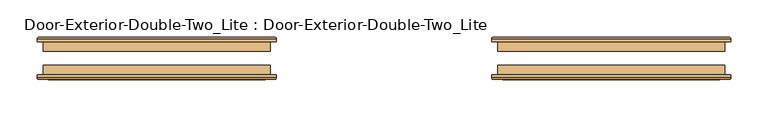
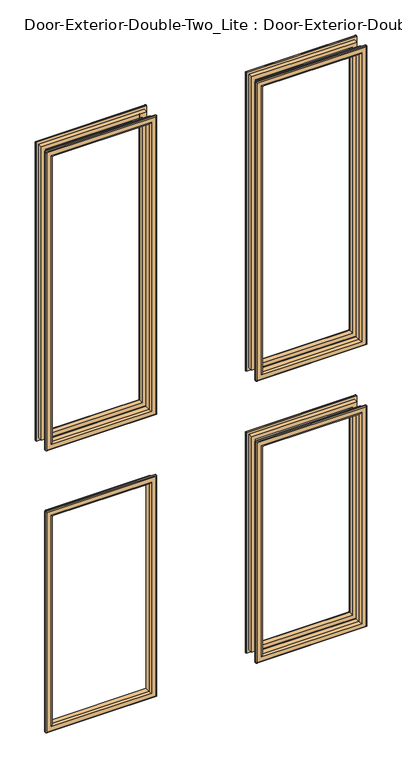
"""IFC4 building model written with IfcOpenShell, lengths in millimetres: door geometry, Door-Exterior-Double-Two_Lite : Door-Exterior-Double-Two_Lite."""

from ifc_helpers import new_model, si_unit, frame, origin, place, context, project, spatial, ellipse_curve, source, transform, mapped, element, save
from ifc_brep_helpers import plane_surface, cylinder_surface, advanced_brep


def door_exterior_double_two_lite_door_exterior_double_two_lite_31e28e64(model_context):
    return source(origin(), model_context, "Body", "AdvancedBrep", [
        advanced_brep(
        [(-457.2, 63.5, 1117.6), (-457.2, 50.8, 1117.6), (-457.2, 50.8, 2016.125), (-457.2, 63.5, 2016.125), (-445.2, 49.8, 1129.6), (-445.2, 63.5, 1129.6), (-445.2, 63.5, 2004.125), (-445.2, 49.8, 2004.125), (-450.2, 44.8, 1124.6), (-450.2, 44.8, 2009.125), (-465.2, 46.8, 1109.6), (-463.2, 44.8, 1111.6), (-463.2, 44.8, 2022.125), (-465.2, 46.8, 2024.125), (-465.2, 50.8, 1109.6), (-465.2, 50.8, 2024.125), (-152.4, 50.8, 2016.125), (-152.4, 63.5, 2016.125), (-164.4, 63.5, 2004.125), (-164.4, 49.8, 2004.125), (-159.4, 44.8, 2009.125), (-146.4, 44.8, 2022.125), (-144.4, 46.8, 2024.125), (-144.4, 50.8, 2024.125), (-152.4, 50.8, 1117.6), (-152.4, 63.5, 1117.6), (-164.4, 63.5, 1129.6), (-164.4, 49.8, 1129.6), (-159.4, 44.8, 1124.6), (-146.4, 44.8, 1111.6), (-144.4, 46.8, 1109.6), (-144.4, 50.8, 1109.6)],
        [
            (0, 1),
            (1, 2),
            (2, 3),
            (3, 0),
            (4, 5),
            (5, 6),
            (6, 7),
            (7, 4),
            (8, 4, ellipse_curve(frame((-450.2, 49.8, 1124.6), z_axis=(-0.7071067811865475, 0.0, 0.7071067811865475), x_axis=(-0.7071067811865474, 0.0, -0.7071067811865476)), 7.0710678, 5.0)),
            (7, 9, ellipse_curve(frame((-450.2, 49.8, 2009.125), z_axis=(-0.7071067811865475, 0.0, -0.7071067811865475), x_axis=(0.7071067811865474, 0.0, -0.7071067811865476)), 7.0710678, 5.0)),
            (9, 8),
            (10, 11, ellipse_curve(frame((-463.2, 46.8, 1111.6), z_axis=(-0.7071067811865475, 0.0, 0.7071067811865475), x_axis=(-0.7071067811865474, 0.0, -0.7071067811865476)), 2.8284271, 2.0)),
            (11, 12),
            (12, 13, ellipse_curve(frame((-463.2, 46.8, 2022.125), z_axis=(-0.7071067811865475, 0.0, -0.7071067811865475), x_axis=(0.7071067811865474, 0.0, -0.7071067811865476)), 2.8284271, 2.0)),
            (13, 10),
            (14, 10),
            (13, 15),
            (15, 14),
            (2, 16),
            (16, 17),
            (17, 3),
            (6, 18),
            (18, 19),
            (19, 7),
            (19, 20, ellipse_curve(frame((-159.4, 49.8, 2009.125), z_axis=(-0.7071067811865475, 0.0, 0.7071067811865475), x_axis=(-0.7071067811865476, 0.0, -0.7071067811865474)), 7.0710678, 5.0)),
            (20, 9),
            (12, 21),
            (21, 22, ellipse_curve(frame((-146.4, 46.8, 2022.125), z_axis=(-0.7071067811865475, 0.0, 0.7071067811865475), x_axis=(-0.7071067811865476, 0.0, -0.7071067811865474)), 2.8284271, 2.0)),
            (22, 13),
            (22, 23),
            (23, 15),
            (16, 24),
            (24, 25),
            (25, 17),
            (18, 26),
            (26, 27),
            (27, 19),
            (27, 28, ellipse_curve(frame((-159.4, 49.8, 1124.6), z_axis=(0.7071067811865475, 0.0, 0.7071067811865475), x_axis=(-0.7071067811865474, 0.0, 0.7071067811865476)), 7.0710678, 5.0)),
            (28, 20),
            (21, 29),
            (29, 30, ellipse_curve(frame((-146.4, 46.8, 1111.6), z_axis=(0.7071067811865475, 0.0, 0.7071067811865475), x_axis=(-0.7071067811865474, 0.0, 0.7071067811865476)), 2.8284271, 2.0)),
            (30, 22),
            (30, 31),
            (31, 23),
            (31, 14),
            (1, 24),
            (0, 25),
            (5, 26),
            (4, 27),
            (8, 28),
            (11, 29),
            (10, 30),
        ],
        [
            plane_surface(frame((-457.2, 50.8, 1117.6), z_axis=(-1.0, 0.0, 0.0), x_axis=(0.0, 0.0, 1.0))),
            plane_surface(frame((-445.2, 63.5, 1129.6), z_axis=(1.0, 0.0, 0.0), x_axis=(0.0, 0.0, 1.0))),
            cylinder_surface(frame((-450.2, 49.8, 1117.6), z_axis=(0.0, 0.0, -1.0), x_axis=(-1.0, 0.0, 0.0)), 5.0),
            cylinder_surface(frame((-463.2, 46.8, 1117.6), z_axis=(0.0, 0.0, -1.0), x_axis=(-1.0, 0.0, 0.0)), 2.0),
            plane_surface(frame((-465.2, 46.8, 1109.6), z_axis=(-1.0, 0.0, 0.0), x_axis=(0.0, 0.0, 1.0))),
            plane_surface(frame((-457.2, 50.8, 2016.125), z_axis=(0.0, 0.0, 1.0), x_axis=(1.0, 0.0, 0.0))),
            plane_surface(frame((-445.2, 63.5, 2004.125), z_axis=(0.0, 0.0, -1.0), x_axis=(1.0, 0.0, 0.0))),
            cylinder_surface(frame((-457.2, 49.8, 2009.125), z_axis=(-1.0, 0.0, 0.0), x_axis=(0.0, 0.0, 1.0)), 5.0),
            cylinder_surface(frame((-457.2, 46.8, 2022.125), z_axis=(-1.0, 0.0, 0.0), x_axis=(0.0, 0.0, 1.0)), 2.0),
            plane_surface(frame((-465.2, 46.8, 2024.125), z_axis=(0.0, 0.0, 1.0), x_axis=(1.0, 0.0, 0.0))),
            plane_surface(frame((-152.4, 50.8, 2016.125), z_axis=(1.0, 0.0, 0.0), x_axis=(0.0, 0.0, -1.0))),
            plane_surface(frame((-164.4, 63.5, 2004.125), z_axis=(-1.0, 0.0, 0.0), x_axis=(0.0, 0.0, -1.0))),
            cylinder_surface(frame((-159.4, 49.8, 2016.125), z_axis=(0.0, 0.0, 1.0), x_axis=(1.0, 0.0, 0.0)), 5.0),
            cylinder_surface(frame((-146.4, 46.8, 2016.125), z_axis=(0.0, 0.0, 1.0), x_axis=(1.0, 0.0, 0.0)), 2.0),
            plane_surface(frame((-144.4, 46.8, 2024.125), z_axis=(1.0, 0.0, 0.0), x_axis=(0.0, 0.0, -1.0))),
            plane_surface(frame((-144.4, 50.8, 1109.6), z_axis=(0.0, 1.0, 0.0), x_axis=(-1.0, 0.0, 0.0))),
            plane_surface(frame((-152.4, 50.8, 1117.6), z_axis=(0.0, 0.0, -1.0), x_axis=(-1.0, 0.0, 0.0))),
            plane_surface(frame((-152.4, 63.5, 1117.6), z_axis=(0.0, 1.0, 0.0), x_axis=(-1.0, 0.0, 0.0))),
            plane_surface(frame((-164.4, 63.5, 1129.6), z_axis=(0.0, 0.0, 1.0), x_axis=(-1.0, 0.0, 0.0))),
            cylinder_surface(frame((-152.4, 49.8, 1124.6), z_axis=(1.0, 0.0, 0.0), x_axis=(0.0, 0.0, -1.0)), 5.0),
            plane_surface(frame((-159.4, 44.8, 1124.6), z_axis=(0.0, -1.0, 0.0), x_axis=(-1.0, 0.0, 0.0))),
            cylinder_surface(frame((-152.4, 46.8, 1111.6), z_axis=(1.0, 0.0, 0.0), x_axis=(0.0, 0.0, -1.0)), 2.0),
            plane_surface(frame((-144.4, 46.8, 1109.6), z_axis=(0.0, 0.0, -1.0), x_axis=(-1.0, 0.0, 0.0))),
        ],
        [
            (0, [[1, 2, 3, 4]]),
            (1, [[5, 6, 7, 8]]),
            (2, [[9, -8, 10, 11]]),
            (3, [[12, 13, 14, 15]]),
            (4, [[16, -15, 17, 18]]),
            (5, [[-3, 19, 20, 21]]),
            (6, [[-7, 22, 23, 24]]),
            (7, [[-10, -24, 25, 26]]),
            (8, [[-14, 27, 28, 29]]),
            (9, [[-17, -29, 30, 31]]),
            (10, [[-20, 32, 33, 34]]),
            (11, [[-23, 35, 36, 37]]),
            (12, [[-25, -37, 38, 39]]),
            (13, [[-28, 40, 41, 42]]),
            (14, [[-30, -42, 43, 44]]),
            (15, [[-31, -44, 45, -18], [46, -32, -19, -2]]),
            (16, [[-33, -46, -1, 47]]),
            (17, [[-21, -34, -47, -4], [48, -35, -22, -6]]),
            (18, [[-36, -48, -5, 49]]),
            (19, [[-38, -49, -9, 50]]),
            (20, [[51, -40, -27, -13], [-26, -39, -50, -11]]),
            (21, [[-41, -51, -12, 52]]),
            (22, [[-43, -52, -16, -45]]),
        ],
    ),
        advanced_brep(
        [(152.4, 63.5, 1117.6), (152.4, 50.8, 1117.6), (152.4, 50.8, 2016.125), (152.4, 63.5, 2016.125), (164.4, 49.8, 1129.6), (164.4, 63.5, 1129.6), (164.4, 63.5, 2004.125), (164.4, 49.8, 2004.125), (159.4, 44.8, 1124.6), (159.4, 44.8, 2009.125), (144.4, 46.8, 1109.6), (146.4, 44.8, 1111.6), (146.4, 44.8, 2022.125), (144.4, 46.8, 2024.125), (144.4, 50.8, 1109.6), (144.4, 50.8, 2024.125), (457.2, 50.8, 2016.125), (457.2, 63.5, 2016.125), (445.2, 63.5, 2004.125), (445.2, 49.8, 2004.125), (450.2, 44.8, 2009.125), (463.2, 44.8, 2022.125), (465.2, 46.8, 2024.125), (465.2, 50.8, 2024.125), (457.2, 50.8, 1117.6), (457.2, 63.5, 1117.6), (445.2, 63.5, 1129.6), (445.2, 49.8, 1129.6), (450.2, 44.8, 1124.6), (463.2, 44.8, 1111.6), (465.2, 46.8, 1109.6), (465.2, 50.8, 1109.6)],
        [
            (0, 1),
            (1, 2),
            (2, 3),
            (3, 0),
            (4, 5),
            (5, 6),
            (6, 7),
            (7, 4),
            (8, 4, ellipse_curve(frame((159.4, 49.8, 1124.6), z_axis=(-0.7071067811865475, 0.0, 0.7071067811865475), x_axis=(-0.7071067811865474, 0.0, -0.7071067811865476)), 7.0710678, 5.0)),
            (7, 9, ellipse_curve(frame((159.4, 49.8, 2009.125), z_axis=(-0.7071067811865475, 0.0, -0.7071067811865475), x_axis=(0.7071067811865474, 0.0, -0.7071067811865476)), 7.0710678, 5.0)),
            (9, 8),
            (10, 11, ellipse_curve(frame((146.4, 46.8, 1111.6), z_axis=(-0.7071067811865475, 0.0, 0.7071067811865475), x_axis=(-0.7071067811865474, 0.0, -0.7071067811865476)), 2.8284271, 2.0)),
            (11, 12),
            (12, 13, ellipse_curve(frame((146.4, 46.8, 2022.125), z_axis=(-0.7071067811865475, 0.0, -0.7071067811865475), x_axis=(0.7071067811865474, 0.0, -0.7071067811865476)), 2.8284271, 2.0)),
            (13, 10),
            (14, 10),
            (13, 15),
            (15, 14),
            (2, 16),
            (16, 17),
            (17, 3),
            (6, 18),
            (18, 19),
            (19, 7),
            (19, 20, ellipse_curve(frame((450.2, 49.8, 2009.125), z_axis=(-0.7071067811865475, 0.0, 0.7071067811865475), x_axis=(-0.7071067811865476, 0.0, -0.7071067811865474)), 7.0710678, 5.0)),
            (20, 9),
            (12, 21),
            (21, 22, ellipse_curve(frame((463.2, 46.8, 2022.125), z_axis=(-0.7071067811865475, 0.0, 0.7071067811865475), x_axis=(-0.7071067811865476, 0.0, -0.7071067811865474)), 2.8284271, 2.0)),
            (22, 13),
            (22, 23),
            (23, 15),
            (16, 24),
            (24, 25),
            (25, 17),
            (18, 26),
            (26, 27),
            (27, 19),
            (27, 28, ellipse_curve(frame((450.2, 49.8, 1124.6), z_axis=(0.7071067811865475, 0.0, 0.7071067811865475), x_axis=(-0.7071067811865474, 0.0, 0.7071067811865476)), 7.0710678, 5.0)),
            (28, 20),
            (21, 29),
            (29, 30, ellipse_curve(frame((463.2, 46.8, 1111.6), z_axis=(0.7071067811865475, 0.0, 0.7071067811865475), x_axis=(-0.7071067811865474, 0.0, 0.7071067811865476)), 2.8284271, 2.0)),
            (30, 22),
            (30, 31),
            (31, 23),
            (31, 14),
            (1, 24),
            (0, 25),
            (5, 26),
            (4, 27),
            (8, 28),
            (11, 29),
            (10, 30),
        ],
        [
            plane_surface(frame((152.4, 50.8, 1117.6), z_axis=(-1.0, 0.0, 0.0), x_axis=(0.0, 0.0, 1.0))),
            plane_surface(frame((164.4, 63.5, 1129.6), z_axis=(1.0, 0.0, 0.0), x_axis=(0.0, 0.0, 1.0))),
            cylinder_surface(frame((159.4, 49.8, 1117.6), z_axis=(0.0, 0.0, -1.0), x_axis=(-1.0, 0.0, 0.0)), 5.0),
            cylinder_surface(frame((146.4, 46.8, 1117.6), z_axis=(0.0, 0.0, -1.0), x_axis=(-1.0, 0.0, 0.0)), 2.0),
            plane_surface(frame((144.4, 46.8, 1109.6), z_axis=(-1.0, 0.0, 0.0), x_axis=(0.0, 0.0, 1.0))),
            plane_surface(frame((152.4, 50.8, 2016.125), z_axis=(0.0, 0.0, 1.0), x_axis=(1.0, 0.0, 0.0))),
            plane_surface(frame((164.4, 63.5, 2004.125), z_axis=(0.0, 0.0, -1.0), x_axis=(1.0, 0.0, 0.0))),
            cylinder_surface(frame((152.4, 49.8, 2009.125), z_axis=(-1.0, 0.0, 0.0), x_axis=(0.0, 0.0, 1.0)), 5.0),
            cylinder_surface(frame((152.4, 46.8, 2022.125), z_axis=(-1.0, 0.0, 0.0), x_axis=(0.0, 0.0, 1.0)), 2.0),
            plane_surface(frame((144.4, 46.8, 2024.125), z_axis=(0.0, 0.0, 1.0), x_axis=(1.0, 0.0, 0.0))),
            plane_surface(frame((457.2, 50.8, 2016.125), z_axis=(1.0, 0.0, 0.0), x_axis=(0.0, 0.0, -1.0))),
            plane_surface(frame((445.2, 63.5, 2004.125), z_axis=(-1.0, 0.0, 0.0), x_axis=(0.0, 0.0, -1.0))),
            cylinder_surface(frame((450.2, 49.8, 2016.125), z_axis=(0.0, 0.0, 1.0), x_axis=(1.0, 0.0, 0.0)), 5.0),
            cylinder_surface(frame((463.2, 46.8, 2016.125), z_axis=(0.0, 0.0, 1.0), x_axis=(1.0, 0.0, 0.0)), 2.0),
            plane_surface(frame((465.2, 46.8, 2024.125), z_axis=(1.0, 0.0, 0.0), x_axis=(0.0, 0.0, -1.0))),
            plane_surface(frame((465.2, 50.8, 1109.6), z_axis=(0.0, 1.0, 0.0), x_axis=(-1.0, 0.0, 0.0))),
            plane_surface(frame((457.2, 50.8, 1117.6), z_axis=(0.0, 0.0, -1.0), x_axis=(-1.0, 0.0, 0.0))),
            plane_surface(frame((457.2, 63.5, 1117.6), z_axis=(0.0, 1.0, 0.0), x_axis=(-1.0, 0.0, 0.0))),
            plane_surface(frame((445.2, 63.5, 1129.6), z_axis=(0.0, 0.0, 1.0), x_axis=(-1.0, 0.0, 0.0))),
            cylinder_surface(frame((457.2, 49.8, 1124.6), z_axis=(1.0, 0.0, 0.0), x_axis=(0.0, 0.0, -1.0)), 5.0),
            plane_surface(frame((450.2, 44.8, 1124.6), z_axis=(0.0, -1.0, 0.0), x_axis=(-1.0, 0.0, 0.0))),
            cylinder_surface(frame((457.2, 46.8, 1111.6), z_axis=(1.0, 0.0, 0.0), x_axis=(0.0, 0.0, -1.0)), 2.0),
            plane_surface(frame((465.2, 46.8, 1109.6), z_axis=(0.0, 0.0, -1.0), x_axis=(-1.0, 0.0, 0.0))),
        ],
        [
            (0, [[1, 2, 3, 4]]),
            (1, [[5, 6, 7, 8]]),
            (2, [[9, -8, 10, 11]]),
            (3, [[12, 13, 14, 15]]),
            (4, [[16, -15, 17, 18]]),
            (5, [[-3, 19, 20, 21]]),
            (6, [[-7, 22, 23, 24]]),
            (7, [[-10, -24, 25, 26]]),
            (8, [[-14, 27, 28, 29]]),
            (9, [[-17, -29, 30, 31]]),
            (10, [[-20, 32, 33, 34]]),
            (11, [[-23, 35, 36, 37]]),
            (12, [[-25, -37, 38, 39]]),
            (13, [[-28, 40, 41, 42]]),
            (14, [[-30, -42, 43, 44]]),
            (15, [[-31, -44, 45, -18], [46, -32, -19, -2]]),
            (16, [[-33, -46, -1, 47]]),
            (17, [[-21, -34, -47, -4], [48, -35, -22, -6]]),
            (18, [[-36, -48, -5, 49]]),
            (19, [[-38, -49, -9, 50]]),
            (20, [[51, -40, -27, -13], [-26, -39, -50, -11]]),
            (21, [[-41, -51, -12, 52]]),
            (22, [[-43, -52, -16, -45]]),
        ],
    ),
        advanced_brep(
        [(152.4, 63.5, 254.0), (152.4, 50.8, 254.0), (152.4, 50.8, 914.4), (152.4, 63.5, 914.4), (164.4, 49.8, 266.0), (164.4, 63.5, 266.0), (164.4, 63.5, 902.4), (164.4, 49.8, 902.4), (159.4, 44.8, 261.0), (159.4, 44.8, 907.4), (144.4, 46.8, 246.0), (146.4, 44.8, 248.0), (146.4, 44.8, 920.4), (144.4, 46.8, 922.4), (144.4, 50.8, 246.0), (144.4, 50.8, 922.4), (457.2, 50.8, 914.4), (457.2, 63.5, 914.4), (445.2, 63.5, 902.4), (445.2, 49.8, 902.4), (450.2, 44.8, 907.4), (463.2, 44.8, 920.4), (465.2, 46.8, 922.4), (465.2, 50.8, 922.4), (457.2, 50.8, 254.0), (457.2, 63.5, 254.0), (445.2, 63.5, 266.0), (445.2, 49.8, 266.0), (450.2, 44.8, 261.0), (463.2, 44.8, 248.0), (465.2, 46.8, 246.0), (465.2, 50.8, 246.0)],
        [
            (0, 1),
            (1, 2),
            (2, 3),
            (3, 0),
            (4, 5),
            (5, 6),
            (6, 7),
            (7, 4),
            (8, 4, ellipse_curve(frame((159.4, 49.8, 261.0), z_axis=(-0.7071067811865475, 0.0, 0.7071067811865475), x_axis=(-0.7071067811865474, 0.0, -0.7071067811865476)), 7.0710678, 5.0)),
            (7, 9, ellipse_curve(frame((159.4, 49.8, 907.4), z_axis=(-0.7071067811865475, 0.0, -0.7071067811865475), x_axis=(0.7071067811865474, 0.0, -0.7071067811865476)), 7.0710678, 5.0)),
            (9, 8),
            (10, 11, ellipse_curve(frame((146.4, 46.8, 248.0), z_axis=(-0.7071067811865475, 0.0, 0.7071067811865475), x_axis=(-0.7071067811865474, 0.0, -0.7071067811865476)), 2.8284271, 2.0)),
            (11, 12),
            (12, 13, ellipse_curve(frame((146.4, 46.8, 920.4), z_axis=(-0.7071067811865475, 0.0, -0.7071067811865475), x_axis=(0.7071067811865474, 0.0, -0.7071067811865476)), 2.8284271, 2.0)),
            (13, 10),
            (14, 10),
            (13, 15),
            (15, 14),
            (2, 16),
            (16, 17),
            (17, 3),
            (6, 18),
            (18, 19),
            (19, 7),
            (19, 20, ellipse_curve(frame((450.2, 49.8, 907.4), z_axis=(-0.7071067811865475, 0.0, 0.7071067811865475), x_axis=(-0.7071067811865476, 0.0, -0.7071067811865474)), 7.0710678, 5.0)),
            (20, 9),
            (12, 21),
            (21, 22, ellipse_curve(frame((463.2, 46.8, 920.4), z_axis=(-0.7071067811865475, 0.0, 0.7071067811865475), x_axis=(-0.7071067811865476, 0.0, -0.7071067811865474)), 2.8284271, 2.0)),
            (22, 13),
            (22, 23),
            (23, 15),
            (16, 24),
            (24, 25),
            (25, 17),
            (18, 26),
            (26, 27),
            (27, 19),
            (27, 28, ellipse_curve(frame((450.2, 49.8, 261.0), z_axis=(0.7071067811865475, 0.0, 0.7071067811865475), x_axis=(-0.7071067811865474, 0.0, 0.7071067811865476)), 7.0710678, 5.0)),
            (28, 20),
            (21, 29),
            (29, 30, ellipse_curve(frame((463.2, 46.8, 248.0), z_axis=(0.7071067811865475, 0.0, 0.7071067811865475), x_axis=(-0.7071067811865474, 0.0, 0.7071067811865476)), 2.8284271, 2.0)),
            (30, 22),
            (30, 31),
            (31, 23),
            (31, 14),
            (1, 24),
            (0, 25),
            (5, 26),
            (4, 27),
            (8, 28),
            (11, 29),
            (10, 30),
        ],
        [
            plane_surface(frame((152.4, 50.8, 254.0), z_axis=(-1.0, 0.0, 0.0), x_axis=(0.0, 0.0, 1.0))),
            plane_surface(frame((164.4, 63.5, 266.0), z_axis=(1.0, 0.0, 0.0), x_axis=(0.0, 0.0, 1.0))),
            cylinder_surface(frame((159.4, 49.8, 254.0), z_axis=(0.0, 0.0, -1.0), x_axis=(-1.0, 0.0, 0.0)), 5.0),
            cylinder_surface(frame((146.4, 46.8, 254.0), z_axis=(0.0, 0.0, -1.0), x_axis=(-1.0, 0.0, 0.0)), 2.0),
            plane_surface(frame((144.4, 46.8, 246.0), z_axis=(-1.0, 0.0, 0.0), x_axis=(0.0, 0.0, 1.0))),
            plane_surface(frame((152.4, 50.8, 914.4), z_axis=(0.0, 0.0, 1.0), x_axis=(1.0, 0.0, 0.0))),
            plane_surface(frame((164.4, 63.5, 902.4), z_axis=(0.0, 0.0, -1.0), x_axis=(1.0, 0.0, 0.0))),
            cylinder_surface(frame((152.4, 49.8, 907.4), z_axis=(-1.0, 0.0, 0.0), x_axis=(0.0, 0.0, 1.0)), 5.0),
            cylinder_surface(frame((152.4, 46.8, 920.4), z_axis=(-1.0, 0.0, 0.0), x_axis=(0.0, 0.0, 1.0)), 2.0),
            plane_surface(frame((144.4, 46.8, 922.4), z_axis=(0.0, 0.0, 1.0), x_axis=(1.0, 0.0, 0.0))),
            plane_surface(frame((457.2, 50.8, 914.4), z_axis=(1.0, 0.0, 0.0), x_axis=(0.0, 0.0, -1.0))),
            plane_surface(frame((445.2, 63.5, 902.4), z_axis=(-1.0, 0.0, 0.0), x_axis=(0.0, 0.0, -1.0))),
            cylinder_surface(frame((450.2, 49.8, 914.4), z_axis=(0.0, 0.0, 1.0), x_axis=(1.0, 0.0, 0.0)), 5.0),
            cylinder_surface(frame((463.2, 46.8, 914.4), z_axis=(0.0, 0.0, 1.0), x_axis=(1.0, 0.0, 0.0)), 2.0),
            plane_surface(frame((465.2, 46.8, 922.4), z_axis=(1.0, 0.0, 0.0), x_axis=(0.0, 0.0, -1.0))),
            plane_surface(frame((465.2, 50.8, 246.0), z_axis=(0.0, 1.0, 0.0), x_axis=(-1.0, 0.0, 0.0))),
            plane_surface(frame((457.2, 50.8, 254.0), z_axis=(0.0, 0.0, -1.0), x_axis=(-1.0, 0.0, 0.0))),
            plane_surface(frame((457.2, 63.5, 254.0), z_axis=(0.0, 1.0, 0.0), x_axis=(-1.0, 0.0, 0.0))),
            plane_surface(frame((445.2, 63.5, 266.0), z_axis=(0.0, 0.0, 1.0), x_axis=(-1.0, 0.0, 0.0))),
            cylinder_surface(frame((457.2, 49.8, 261.0), z_axis=(1.0, 0.0, 0.0), x_axis=(0.0, 0.0, -1.0)), 5.0),
            plane_surface(frame((450.2, 44.8, 261.0), z_axis=(0.0, -1.0, 0.0), x_axis=(-1.0, 0.0, 0.0))),
            cylinder_surface(frame((457.2, 46.8, 248.0), z_axis=(1.0, 0.0, 0.0), x_axis=(0.0, 0.0, -1.0)), 2.0),
            plane_surface(frame((465.2, 46.8, 246.0), z_axis=(0.0, 0.0, -1.0), x_axis=(-1.0, 0.0, 0.0))),
        ],
        [
            (0, [[1, 2, 3, 4]]),
            (1, [[5, 6, 7, 8]]),
            (2, [[9, -8, 10, 11]]),
            (3, [[12, 13, 14, 15]]),
            (4, [[16, -15, 17, 18]]),
            (5, [[-3, 19, 20, 21]]),
            (6, [[-7, 22, 23, 24]]),
            (7, [[-10, -24, 25, 26]]),
            (8, [[-14, 27, 28, 29]]),
            (9, [[-17, -29, 30, 31]]),
            (10, [[-20, 32, 33, 34]]),
            (11, [[-23, 35, 36, 37]]),
            (12, [[-25, -37, 38, 39]]),
            (13, [[-28, 40, 41, 42]]),
            (14, [[-30, -42, 43, 44]]),
            (15, [[-31, -44, 45, -18], [46, -32, -19, -2]]),
            (16, [[-33, -46, -1, 47]]),
            (17, [[-21, -34, -47, -4], [48, -35, -22, -6]]),
            (18, [[-36, -48, -5, 49]]),
            (19, [[-38, -49, -9, 50]]),
            (20, [[51, -40, -27, -13], [-26, -39, -50, -11]]),
            (21, [[-41, -51, -12, 52]]),
            (22, [[-43, -52, -16, -45]]),
        ],
    ),
        advanced_brep(
        [(-457.2, 63.5, 254.0), (-457.2, 50.8, 254.0), (-457.2, 50.8, 914.4), (-457.2, 63.5, 914.4), (-445.2, 49.8, 266.0), (-445.2, 63.5, 266.0), (-445.2, 63.5, 902.4), (-445.2, 49.8, 902.4), (-450.2, 44.8, 261.0), (-450.2, 44.8, 907.4), (-465.2, 46.8, 246.0), (-463.2, 44.8, 248.0), (-463.2, 44.8, 920.4), (-465.2, 46.8, 922.4), (-465.2, 50.8, 246.0), (-465.2, 50.8, 922.4), (-152.4, 50.8, 914.4), (-152.4, 63.5, 914.4), (-164.4, 63.5, 902.4), (-164.4, 49.8, 902.4), (-159.4, 44.8, 907.4), (-146.4, 44.8, 920.4), (-144.4, 46.8, 922.4), (-144.4, 50.8, 922.4), (-152.4, 50.8, 254.0), (-152.4, 63.5, 254.0), (-164.4, 63.5, 266.0), (-164.4, 49.8, 266.0), (-159.4, 44.8, 261.0), (-146.4, 44.8, 248.0), (-144.4, 46.8, 246.0), (-144.4, 50.8, 246.0)],
        [
            (0, 1),
            (1, 2),
            (2, 3),
            (3, 0),
            (4, 5),
            (5, 6),
            (6, 7),
            (7, 4),
            (8, 4, ellipse_curve(frame((-450.2, 49.8, 261.0), z_axis=(-0.7071067811865475, 0.0, 0.7071067811865475), x_axis=(-0.7071067811865474, 0.0, -0.7071067811865476)), 7.0710678, 5.0)),
            (7, 9, ellipse_curve(frame((-450.2, 49.8, 907.4), z_axis=(-0.7071067811865475, 0.0, -0.7071067811865475), x_axis=(0.7071067811865474, 0.0, -0.7071067811865476)), 7.0710678, 5.0)),
            (9, 8),
            (10, 11, ellipse_curve(frame((-463.2, 46.8, 248.0), z_axis=(-0.7071067811865475, 0.0, 0.7071067811865475), x_axis=(-0.7071067811865474, 0.0, -0.7071067811865476)), 2.8284271, 2.0)),
            (11, 12),
            (12, 13, ellipse_curve(frame((-463.2, 46.8, 920.4), z_axis=(-0.7071067811865475, 0.0, -0.7071067811865475), x_axis=(0.7071067811865474, 0.0, -0.7071067811865476)), 2.8284271, 2.0)),
            (13, 10),
            (14, 10),
            (13, 15),
            (15, 14),
            (2, 16),
            (16, 17),
            (17, 3),
            (6, 18),
            (18, 19),
            (19, 7),
            (19, 20, ellipse_curve(frame((-159.4, 49.8, 907.4), z_axis=(-0.7071067811865475, 0.0, 0.7071067811865475), x_axis=(-0.7071067811865476, 0.0, -0.7071067811865474)), 7.0710678, 5.0)),
            (20, 9),
            (12, 21),
            (21, 22, ellipse_curve(frame((-146.4, 46.8, 920.4), z_axis=(-0.7071067811865475, 0.0, 0.7071067811865475), x_axis=(-0.7071067811865476, 0.0, -0.7071067811865474)), 2.8284271, 2.0)),
            (22, 13),
            (22, 23),
            (23, 15),
            (16, 24),
            (24, 25),
            (25, 17),
            (18, 26),
            (26, 27),
            (27, 19),
            (27, 28, ellipse_curve(frame((-159.4, 49.8, 261.0), z_axis=(0.7071067811865475, 0.0, 0.7071067811865475), x_axis=(-0.7071067811865474, 0.0, 0.7071067811865476)), 7.0710678, 5.0)),
            (28, 20),
            (21, 29),
            (29, 30, ellipse_curve(frame((-146.4, 46.8, 248.0), z_axis=(0.7071067811865475, 0.0, 0.7071067811865475), x_axis=(-0.7071067811865474, 0.0, 0.7071067811865476)), 2.8284271, 2.0)),
            (30, 22),
            (30, 31),
            (31, 23),
            (31, 14),
            (1, 24),
            (0, 25),
            (5, 26),
            (4, 27),
            (8, 28),
            (11, 29),
            (10, 30),
        ],
        [
            plane_surface(frame((-457.2, 50.8, 254.0), z_axis=(-1.0, 0.0, 0.0), x_axis=(0.0, 0.0, 1.0))),
            plane_surface(frame((-445.2, 63.5, 266.0), z_axis=(1.0, 0.0, 0.0), x_axis=(0.0, 0.0, 1.0))),
            cylinder_surface(frame((-450.2, 49.8, 254.0), z_axis=(0.0, 0.0, -1.0), x_axis=(-1.0, 0.0, 0.0)), 5.0),
            cylinder_surface(frame((-463.2, 46.8, 254.0), z_axis=(0.0, 0.0, -1.0), x_axis=(-1.0, 0.0, 0.0)), 2.0),
            plane_surface(frame((-465.2, 46.8, 246.0), z_axis=(-1.0, 0.0, 0.0), x_axis=(0.0, 0.0, 1.0))),
            plane_surface(frame((-457.2, 50.8, 914.4), z_axis=(0.0, 0.0, 1.0), x_axis=(1.0, 0.0, 0.0))),
            plane_surface(frame((-445.2, 63.5, 902.4), z_axis=(0.0, 0.0, -1.0), x_axis=(1.0, 0.0, 0.0))),
            cylinder_surface(frame((-457.2, 49.8, 907.4), z_axis=(-1.0, 0.0, 0.0), x_axis=(0.0, 0.0, 1.0)), 5.0),
            cylinder_surface(frame((-457.2, 46.8, 920.4), z_axis=(-1.0, 0.0, 0.0), x_axis=(0.0, 0.0, 1.0)), 2.0),
            plane_surface(frame((-465.2, 46.8, 922.4), z_axis=(0.0, 0.0, 1.0), x_axis=(1.0, 0.0, 0.0))),
            plane_surface(frame((-152.4, 50.8, 914.4), z_axis=(1.0, 0.0, 0.0), x_axis=(0.0, 0.0, -1.0))),
            plane_surface(frame((-164.4, 63.5, 902.4), z_axis=(-1.0, 0.0, 0.0), x_axis=(0.0, 0.0, -1.0))),
            cylinder_surface(frame((-159.4, 49.8, 914.4), z_axis=(0.0, 0.0, 1.0), x_axis=(1.0, 0.0, 0.0)), 5.0),
            cylinder_surface(frame((-146.4, 46.8, 914.4), z_axis=(0.0, 0.0, 1.0), x_axis=(1.0, 0.0, 0.0)), 2.0),
            plane_surface(frame((-144.4, 46.8, 922.4), z_axis=(1.0, 0.0, 0.0), x_axis=(0.0, 0.0, -1.0))),
            plane_surface(frame((-144.4, 50.8, 246.0), z_axis=(0.0, 1.0, 0.0), x_axis=(-1.0, 0.0, 0.0))),
            plane_surface(frame((-152.4, 50.8, 254.0), z_axis=(0.0, 0.0, -1.0), x_axis=(-1.0, 0.0, 0.0))),
            plane_surface(frame((-152.4, 63.5, 254.0), z_axis=(0.0, 1.0, 0.0), x_axis=(-1.0, 0.0, 0.0))),
            plane_surface(frame((-164.4, 63.5, 266.0), z_axis=(0.0, 0.0, 1.0), x_axis=(-1.0, 0.0, 0.0))),
            cylinder_surface(frame((-152.4, 49.8, 261.0), z_axis=(1.0, 0.0, 0.0), x_axis=(0.0, 0.0, -1.0)), 5.0),
            plane_surface(frame((-159.4, 44.8, 261.0), z_axis=(0.0, -1.0, 0.0), x_axis=(-1.0, 0.0, 0.0))),
            cylinder_surface(frame((-152.4, 46.8, 248.0), z_axis=(1.0, 0.0, 0.0), x_axis=(0.0, 0.0, -1.0)), 2.0),
            plane_surface(frame((-144.4, 46.8, 246.0), z_axis=(0.0, 0.0, -1.0), x_axis=(-1.0, 0.0, 0.0))),
        ],
        [
            (0, [[1, 2, 3, 4]]),
            (1, [[5, 6, 7, 8]]),
            (2, [[9, -8, 10, 11]]),
            (3, [[12, 13, 14, 15]]),
            (4, [[16, -15, 17, 18]]),
            (5, [[-3, 19, 20, 21]]),
            (6, [[-7, 22, 23, 24]]),
            (7, [[-10, -24, 25, 26]]),
            (8, [[-14, 27, 28, 29]]),
            (9, [[-17, -29, 30, 31]]),
            (10, [[-20, 32, 33, 34]]),
            (11, [[-23, 35, 36, 37]]),
            (12, [[-25, -37, 38, 39]]),
            (13, [[-28, 40, 41, 42]]),
            (14, [[-30, -42, 43, 44]]),
            (15, [[-31, -44, 45, -18], [46, -32, -19, -2]]),
            (16, [[-33, -46, -1, 47]]),
            (17, [[-21, -34, -47, -4], [48, -35, -22, -6]]),
            (18, [[-36, -48, -5, 49]]),
            (19, [[-38, -49, -9, 50]]),
            (20, [[51, -40, -27, -13], [-26, -39, -50, -11]]),
            (21, [[-41, -51, -12, 52]]),
            (22, [[-43, -52, -16, -45]]),
        ],
    ),
        advanced_brep(
        [(-457.2, 82.55, 2016.125), (-457.2, 95.25, 2016.125), (-457.2, 95.25, 1117.6), (-457.2, 82.55, 1117.6), (-445.2, 96.25, 2004.125), (-445.2, 82.55, 2004.125), (-445.2, 82.55, 1129.6), (-445.2, 96.25, 1129.6), (-450.2, 101.25, 2009.125), (-450.2, 101.25, 1124.6), (-465.2, 99.25, 2024.125), (-463.2, 101.25, 2022.125), (-463.2, 101.25, 1111.6), (-465.2, 99.25, 1109.6), (-465.2, 95.25, 2024.125), (-465.2, 95.25, 1109.6), (-152.4, 95.25, 1117.6), (-152.4, 82.55, 1117.6), (-164.4, 82.55, 1129.6), (-164.4, 96.25, 1129.6), (-159.4, 101.25, 1124.6), (-146.4, 101.25, 1111.6), (-144.4, 99.25, 1109.6), (-144.4, 95.25, 1109.6), (-152.4, 95.25, 2016.125), (-152.4, 82.55, 2016.125), (-164.4, 82.55, 2004.125), (-164.4, 96.25, 2004.125), (-159.4, 101.25, 2009.125), (-146.4, 101.25, 2022.125), (-144.4, 99.25, 2024.125), (-144.4, 95.25, 2024.125)],
        [
            (0, 1),
            (1, 2),
            (2, 3),
            (3, 0),
            (4, 5),
            (5, 6),
            (6, 7),
            (7, 4),
            (8, 4, ellipse_curve(frame((-450.2, 96.25, 2009.125), z_axis=(-0.7071067811865475, 0.0, -0.7071067811865475), x_axis=(-0.7071067811865474, 0.0, 0.7071067811865476)), 7.0710678, 5.0)),
            (7, 9, ellipse_curve(frame((-450.2, 96.25, 1124.6), z_axis=(-0.7071067811865475, 0.0, 0.7071067811865475), x_axis=(0.7071067811865474, 0.0, 0.7071067811865476)), 7.0710678, 5.0)),
            (9, 8),
            (10, 11, ellipse_curve(frame((-463.2, 99.25, 2022.125), z_axis=(-0.7071067811865475, 0.0, -0.7071067811865475), x_axis=(-0.7071067811865474, 0.0, 0.7071067811865476)), 2.8284271, 2.0)),
            (11, 12),
            (12, 13, ellipse_curve(frame((-463.2, 99.25, 1111.6), z_axis=(-0.7071067811865475, 0.0, 0.7071067811865475), x_axis=(0.7071067811865474, 0.0, 0.7071067811865476)), 2.8284271, 2.0)),
            (13, 10),
            (14, 10),
            (13, 15),
            (15, 14),
            (2, 16),
            (16, 17),
            (17, 3),
            (6, 18),
            (18, 19),
            (19, 7),
            (19, 20, ellipse_curve(frame((-159.4, 96.25, 1124.6), z_axis=(-0.7071067811865475, 0.0, -0.7071067811865475), x_axis=(-0.7071067811865476, 0.0, 0.7071067811865474)), 7.0710678, 5.0)),
            (20, 9),
            (12, 21),
            (21, 22, ellipse_curve(frame((-146.4, 99.25, 1111.6), z_axis=(-0.7071067811865475, 0.0, -0.7071067811865475), x_axis=(-0.7071067811865476, 0.0, 0.7071067811865474)), 2.8284271, 2.0)),
            (22, 13),
            (22, 23),
            (23, 15),
            (16, 24),
            (24, 25),
            (25, 17),
            (18, 26),
            (26, 27),
            (27, 19),
            (27, 28, ellipse_curve(frame((-159.4, 96.25, 2009.125), z_axis=(0.7071067811865475, 0.0, -0.7071067811865475), x_axis=(-0.7071067811865474, 0.0, -0.7071067811865476)), 7.0710678, 5.0)),
            (28, 20),
            (21, 29),
            (29, 30, ellipse_curve(frame((-146.4, 99.25, 2022.125), z_axis=(0.7071067811865475, 0.0, -0.7071067811865475), x_axis=(-0.7071067811865474, 0.0, -0.7071067811865476)), 2.8284271, 2.0)),
            (30, 22),
            (30, 31),
            (31, 23),
            (31, 14),
            (1, 24),
            (0, 25),
            (5, 26),
            (4, 27),
            (8, 28),
            (11, 29),
            (10, 30),
        ],
        [
            plane_surface(frame((-457.2, 95.25, 2016.125), z_axis=(-1.0, 0.0, 0.0), x_axis=(0.0, 0.0, -1.0))),
            plane_surface(frame((-445.2, 82.55, 2004.125), z_axis=(1.0, 0.0, 0.0), x_axis=(0.0, 0.0, -1.0))),
            cylinder_surface(frame((-450.2, 96.25, 2016.125), z_axis=(0.0, 0.0, 1.0), x_axis=(-1.0, 0.0, 0.0)), 5.0),
            cylinder_surface(frame((-463.2, 99.25, 2016.125), z_axis=(0.0, 0.0, 1.0), x_axis=(-1.0, 0.0, 0.0)), 2.0),
            plane_surface(frame((-465.2, 99.25, 2024.125), z_axis=(-1.0, 0.0, 0.0), x_axis=(0.0, 0.0, -1.0))),
            plane_surface(frame((-457.2, 95.25, 1117.6), z_axis=(0.0, 0.0, -1.0), x_axis=(1.0, 0.0, 0.0))),
            plane_surface(frame((-445.2, 82.55, 1129.6), z_axis=(0.0, 0.0, 1.0), x_axis=(1.0, 0.0, 0.0))),
            cylinder_surface(frame((-457.2, 96.25, 1124.6), z_axis=(-1.0, 0.0, 0.0), x_axis=(0.0, 0.0, -1.0)), 5.0),
            cylinder_surface(frame((-457.2, 99.25, 1111.6), z_axis=(-1.0, 0.0, 0.0), x_axis=(0.0, 0.0, -1.0)), 2.0),
            plane_surface(frame((-465.2, 99.25, 1109.6), z_axis=(0.0, 0.0, -1.0), x_axis=(1.0, 0.0, 0.0))),
            plane_surface(frame((-152.4, 95.25, 1117.6), z_axis=(1.0, 0.0, 0.0), x_axis=(0.0, 0.0, 1.0))),
            plane_surface(frame((-164.4, 82.55, 1129.6), z_axis=(-1.0, 0.0, 0.0), x_axis=(0.0, 0.0, 1.0))),
            cylinder_surface(frame((-159.4, 96.25, 1117.6), z_axis=(0.0, 0.0, -1.0), x_axis=(1.0, 0.0, 0.0)), 5.0),
            cylinder_surface(frame((-146.4, 99.25, 1117.6), z_axis=(0.0, 0.0, -1.0), x_axis=(1.0, 0.0, 0.0)), 2.0),
            plane_surface(frame((-144.4, 99.25, 1109.6), z_axis=(1.0, 0.0, 0.0), x_axis=(0.0, 0.0, 1.0))),
            plane_surface(frame((-144.4, 95.25, 2024.125), z_axis=(0.0, -1.0, 0.0), x_axis=(-1.0, 0.0, 0.0))),
            plane_surface(frame((-152.4, 95.25, 2016.125), z_axis=(0.0, 0.0, 1.0), x_axis=(-1.0, 0.0, 0.0))),
            plane_surface(frame((-152.4, 82.55, 2016.125), z_axis=(0.0, -1.0, 0.0), x_axis=(-1.0, 0.0, 0.0))),
            plane_surface(frame((-164.4, 82.55, 2004.125), z_axis=(0.0, 0.0, -1.0), x_axis=(-1.0, 0.0, 0.0))),
            cylinder_surface(frame((-152.4, 96.25, 2009.125), z_axis=(1.0, 0.0, 0.0), x_axis=(0.0, 0.0, 1.0)), 5.0),
            plane_surface(frame((-159.4, 101.25, 2009.125), z_axis=(0.0, 1.0, 0.0), x_axis=(-1.0, 0.0, 0.0))),
            cylinder_surface(frame((-152.4, 99.25, 2022.125), z_axis=(1.0, 0.0, 0.0), x_axis=(0.0, 0.0, 1.0)), 2.0),
            plane_surface(frame((-144.4, 99.25, 2024.125), z_axis=(0.0, 0.0, 1.0), x_axis=(-1.0, 0.0, 0.0))),
        ],
        [
            (0, [[1, 2, 3, 4]]),
            (1, [[5, 6, 7, 8]]),
            (2, [[9, -8, 10, 11]]),
            (3, [[12, 13, 14, 15]]),
            (4, [[16, -15, 17, 18]]),
            (5, [[-3, 19, 20, 21]]),
            (6, [[-7, 22, 23, 24]]),
            (7, [[-10, -24, 25, 26]]),
            (8, [[-14, 27, 28, 29]]),
            (9, [[-17, -29, 30, 31]]),
            (10, [[-20, 32, 33, 34]]),
            (11, [[-23, 35, 36, 37]]),
            (12, [[-25, -37, 38, 39]]),
            (13, [[-28, 40, 41, 42]]),
            (14, [[-30, -42, 43, 44]]),
            (15, [[-31, -44, 45, -18], [46, -32, -19, -2]]),
            (16, [[-33, -46, -1, 47]]),
            (17, [[-21, -34, -47, -4], [48, -35, -22, -6]]),
            (18, [[-36, -48, -5, 49]]),
            (19, [[-38, -49, -9, 50]]),
            (20, [[51, -40, -27, -13], [-26, -39, -50, -11]]),
            (21, [[-41, -51, -12, 52]]),
            (22, [[-43, -52, -16, -45]]),
        ],
    ),
        advanced_brep(
        [(152.4, 82.55, 2016.125), (152.4, 95.25, 2016.125), (152.4, 95.25, 1117.6), (152.4, 82.55, 1117.6), (164.4, 96.25, 2004.125), (164.4, 82.55, 2004.125), (164.4, 82.55, 1129.6), (164.4, 96.25, 1129.6), (159.4, 101.25, 2009.125), (159.4, 101.25, 1124.6), (144.4, 99.25, 2024.125), (146.4, 101.25, 2022.125), (146.4, 101.25, 1111.6), (144.4, 99.25, 1109.6), (144.4, 95.25, 2024.125), (144.4, 95.25, 1109.6), (457.2, 95.25, 1117.6), (457.2, 82.55, 1117.6), (445.2, 82.55, 1129.6), (445.2, 96.25, 1129.6), (450.2, 101.25, 1124.6), (463.2, 101.25, 1111.6), (465.2, 99.25, 1109.6), (465.2, 95.25, 1109.6), (457.2, 95.25, 2016.125), (457.2, 82.55, 2016.125), (445.2, 82.55, 2004.125), (445.2, 96.25, 2004.125), (450.2, 101.25, 2009.125), (463.2, 101.25, 2022.125), (465.2, 99.25, 2024.125), (465.2, 95.25, 2024.125)],
        [
            (0, 1),
            (1, 2),
            (2, 3),
            (3, 0),
            (4, 5),
            (5, 6),
            (6, 7),
            (7, 4),
            (8, 4, ellipse_curve(frame((159.4, 96.25, 2009.125), z_axis=(-0.7071067811865475, 0.0, -0.7071067811865475), x_axis=(-0.7071067811865474, 0.0, 0.7071067811865476)), 7.0710678, 5.0)),
            (7, 9, ellipse_curve(frame((159.4, 96.25, 1124.6), z_axis=(-0.7071067811865475, 0.0, 0.7071067811865475), x_axis=(0.7071067811865474, 0.0, 0.7071067811865476)), 7.0710678, 5.0)),
            (9, 8),
            (10, 11, ellipse_curve(frame((146.4, 99.25, 2022.125), z_axis=(-0.7071067811865475, 0.0, -0.7071067811865475), x_axis=(-0.7071067811865474, 0.0, 0.7071067811865476)), 2.8284271, 2.0)),
            (11, 12),
            (12, 13, ellipse_curve(frame((146.4, 99.25, 1111.6), z_axis=(-0.7071067811865475, 0.0, 0.7071067811865475), x_axis=(0.7071067811865474, 0.0, 0.7071067811865476)), 2.8284271, 2.0)),
            (13, 10),
            (14, 10),
            (13, 15),
            (15, 14),
            (2, 16),
            (16, 17),
            (17, 3),
            (6, 18),
            (18, 19),
            (19, 7),
            (19, 20, ellipse_curve(frame((450.2, 96.25, 1124.6), z_axis=(-0.7071067811865475, 0.0, -0.7071067811865475), x_axis=(-0.7071067811865476, 0.0, 0.7071067811865474)), 7.0710678, 5.0)),
            (20, 9),
            (12, 21),
            (21, 22, ellipse_curve(frame((463.2, 99.25, 1111.6), z_axis=(-0.7071067811865475, 0.0, -0.7071067811865475), x_axis=(-0.7071067811865476, 0.0, 0.7071067811865474)), 2.8284271, 2.0)),
            (22, 13),
            (22, 23),
            (23, 15),
            (16, 24),
            (24, 25),
            (25, 17),
            (18, 26),
            (26, 27),
            (27, 19),
            (27, 28, ellipse_curve(frame((450.2, 96.25, 2009.125), z_axis=(0.7071067811865475, 0.0, -0.7071067811865475), x_axis=(-0.7071067811865474, 0.0, -0.7071067811865476)), 7.0710678, 5.0)),
            (28, 20),
            (21, 29),
            (29, 30, ellipse_curve(frame((463.2, 99.25, 2022.125), z_axis=(0.7071067811865475, 0.0, -0.7071067811865475), x_axis=(-0.7071067811865474, 0.0, -0.7071067811865476)), 2.8284271, 2.0)),
            (30, 22),
            (30, 31),
            (31, 23),
            (31, 14),
            (1, 24),
            (0, 25),
            (5, 26),
            (4, 27),
            (8, 28),
            (11, 29),
            (10, 30),
        ],
        [
            plane_surface(frame((152.4, 95.25, 2016.125), z_axis=(-1.0, 0.0, 0.0), x_axis=(0.0, 0.0, -1.0))),
            plane_surface(frame((164.4, 82.55, 2004.125), z_axis=(1.0, 0.0, 0.0), x_axis=(0.0, 0.0, -1.0))),
            cylinder_surface(frame((159.4, 96.25, 2016.125), z_axis=(0.0, 0.0, 1.0), x_axis=(-1.0, 0.0, 0.0)), 5.0),
            cylinder_surface(frame((146.4, 99.25, 2016.125), z_axis=(0.0, 0.0, 1.0), x_axis=(-1.0, 0.0, 0.0)), 2.0),
            plane_surface(frame((144.4, 99.25, 2024.125), z_axis=(-1.0, 0.0, 0.0), x_axis=(0.0, 0.0, -1.0))),
            plane_surface(frame((152.4, 95.25, 1117.6), z_axis=(0.0, 0.0, -1.0), x_axis=(1.0, 0.0, 0.0))),
            plane_surface(frame((164.4, 82.55, 1129.6), z_axis=(0.0, 0.0, 1.0), x_axis=(1.0, 0.0, 0.0))),
            cylinder_surface(frame((152.4, 96.25, 1124.6), z_axis=(-1.0, 0.0, 0.0), x_axis=(0.0, 0.0, -1.0)), 5.0),
            cylinder_surface(frame((152.4, 99.25, 1111.6), z_axis=(-1.0, 0.0, 0.0), x_axis=(0.0, 0.0, -1.0)), 2.0),
            plane_surface(frame((144.4, 99.25, 1109.6), z_axis=(0.0, 0.0, -1.0), x_axis=(1.0, 0.0, 0.0))),
            plane_surface(frame((457.2, 95.25, 1117.6), z_axis=(1.0, 0.0, 0.0), x_axis=(0.0, 0.0, 1.0))),
            plane_surface(frame((445.2, 82.55, 1129.6), z_axis=(-1.0, 0.0, 0.0), x_axis=(0.0, 0.0, 1.0))),
            cylinder_surface(frame((450.2, 96.25, 1117.6), z_axis=(0.0, 0.0, -1.0), x_axis=(1.0, 0.0, 0.0)), 5.0),
            cylinder_surface(frame((463.2, 99.25, 1117.6), z_axis=(0.0, 0.0, -1.0), x_axis=(1.0, 0.0, 0.0)), 2.0),
            plane_surface(frame((465.2, 99.25, 1109.6), z_axis=(1.0, 0.0, 0.0), x_axis=(0.0, 0.0, 1.0))),
            plane_surface(frame((465.2, 95.25, 2024.125), z_axis=(0.0, -1.0, 0.0), x_axis=(-1.0, 0.0, 0.0))),
            plane_surface(frame((457.2, 95.25, 2016.125), z_axis=(0.0, 0.0, 1.0), x_axis=(-1.0, 0.0, 0.0))),
            plane_surface(frame((457.2, 82.55, 2016.125), z_axis=(0.0, -1.0, 0.0), x_axis=(-1.0, 0.0, 0.0))),
            plane_surface(frame((445.2, 82.55, 2004.125), z_axis=(0.0, 0.0, -1.0), x_axis=(-1.0, 0.0, 0.0))),
            cylinder_surface(frame((457.2, 96.25, 2009.125), z_axis=(1.0, 0.0, 0.0), x_axis=(0.0, 0.0, 1.0)), 5.0),
            plane_surface(frame((450.2, 101.25, 2009.125), z_axis=(0.0, 1.0, 0.0), x_axis=(-1.0, 0.0, 0.0))),
            cylinder_surface(frame((457.2, 99.25, 2022.125), z_axis=(1.0, 0.0, 0.0), x_axis=(0.0, 0.0, 1.0)), 2.0),
            plane_surface(frame((465.2, 99.25, 2024.125), z_axis=(0.0, 0.0, 1.0), x_axis=(-1.0, 0.0, 0.0))),
        ],
        [
            (0, [[1, 2, 3, 4]]),
            (1, [[5, 6, 7, 8]]),
            (2, [[9, -8, 10, 11]]),
            (3, [[12, 13, 14, 15]]),
            (4, [[16, -15, 17, 18]]),
            (5, [[-3, 19, 20, 21]]),
            (6, [[-7, 22, 23, 24]]),
            (7, [[-10, -24, 25, 26]]),
            (8, [[-14, 27, 28, 29]]),
            (9, [[-17, -29, 30, 31]]),
            (10, [[-20, 32, 33, 34]]),
            (11, [[-23, 35, 36, 37]]),
            (12, [[-25, -37, 38, 39]]),
            (13, [[-28, 40, 41, 42]]),
            (14, [[-30, -42, 43, 44]]),
            (15, [[-31, -44, 45, -18], [46, -32, -19, -2]]),
            (16, [[-33, -46, -1, 47]]),
            (17, [[-21, -34, -47, -4], [48, -35, -22, -6]]),
            (18, [[-36, -48, -5, 49]]),
            (19, [[-38, -49, -9, 50]]),
            (20, [[51, -40, -27, -13], [-26, -39, -50, -11]]),
            (21, [[-41, -51, -12, 52]]),
            (22, [[-43, -52, -16, -45]]),
        ],
    ),
        advanced_brep(
        [(152.4, 82.55, 914.4), (152.4, 95.25, 914.4), (152.4, 95.25, 254.0), (152.4, 82.55, 254.0), (164.4, 96.25, 902.4), (164.4, 82.55, 902.4), (164.4, 82.55, 266.0), (164.4, 96.25, 266.0), (159.4, 101.25, 907.4), (159.4, 101.25, 261.0), (144.4, 99.25, 922.4), (146.4, 101.25, 920.4), (146.4, 101.25, 248.0), (144.4, 99.25, 246.0), (144.4, 95.25, 922.4), (144.4, 95.25, 246.0), (457.2, 95.25, 254.0), (457.2, 82.55, 254.0), (445.2, 82.55, 266.0), (445.2, 96.25, 266.0), (450.2, 101.25, 261.0), (463.2, 101.25, 248.0), (465.2, 99.25, 246.0), (465.2, 95.25, 246.0), (457.2, 95.25, 914.4), (457.2, 82.55, 914.4), (445.2, 82.55, 902.4), (445.2, 96.25, 902.4), (450.2, 101.25, 907.4), (463.2, 101.25, 920.4), (465.2, 99.25, 922.4), (465.2, 95.25, 922.4)],
        [
            (0, 1),
            (1, 2),
            (2, 3),
            (3, 0),
            (4, 5),
            (5, 6),
            (6, 7),
            (7, 4),
            (8, 4, ellipse_curve(frame((159.4, 96.25, 907.4), z_axis=(-0.7071067811865475, 0.0, -0.7071067811865475), x_axis=(-0.7071067811865474, 0.0, 0.7071067811865476)), 7.0710678, 5.0)),
            (7, 9, ellipse_curve(frame((159.4, 96.25, 261.0), z_axis=(-0.7071067811865475, 0.0, 0.7071067811865475), x_axis=(0.7071067811865474, 0.0, 0.7071067811865476)), 7.0710678, 5.0)),
            (9, 8),
            (10, 11, ellipse_curve(frame((146.4, 99.25, 920.4), z_axis=(-0.7071067811865475, 0.0, -0.7071067811865475), x_axis=(-0.7071067811865474, 0.0, 0.7071067811865476)), 2.8284271, 2.0)),
            (11, 12),
            (12, 13, ellipse_curve(frame((146.4, 99.25, 248.0), z_axis=(-0.7071067811865475, 0.0, 0.7071067811865475), x_axis=(0.7071067811865474, 0.0, 0.7071067811865476)), 2.8284271, 2.0)),
            (13, 10),
            (14, 10),
            (13, 15),
            (15, 14),
            (2, 16),
            (16, 17),
            (17, 3),
            (6, 18),
            (18, 19),
            (19, 7),
            (19, 20, ellipse_curve(frame((450.2, 96.25, 261.0), z_axis=(-0.7071067811865475, 0.0, -0.7071067811865475), x_axis=(-0.7071067811865476, 0.0, 0.7071067811865474)), 7.0710678, 5.0)),
            (20, 9),
            (12, 21),
            (21, 22, ellipse_curve(frame((463.2, 99.25, 248.0), z_axis=(-0.7071067811865475, 0.0, -0.7071067811865475), x_axis=(-0.7071067811865476, 0.0, 0.7071067811865474)), 2.8284271, 2.0)),
            (22, 13),
            (22, 23),
            (23, 15),
            (16, 24),
            (24, 25),
            (25, 17),
            (18, 26),
            (26, 27),
            (27, 19),
            (27, 28, ellipse_curve(frame((450.2, 96.25, 907.4), z_axis=(0.7071067811865475, 0.0, -0.7071067811865475), x_axis=(-0.7071067811865474, 0.0, -0.7071067811865476)), 7.0710678, 5.0)),
            (28, 20),
            (21, 29),
            (29, 30, ellipse_curve(frame((463.2, 99.25, 920.4), z_axis=(0.7071067811865475, 0.0, -0.7071067811865475), x_axis=(-0.7071067811865474, 0.0, -0.7071067811865476)), 2.8284271, 2.0)),
            (30, 22),
            (30, 31),
            (31, 23),
            (31, 14),
            (1, 24),
            (0, 25),
            (5, 26),
            (4, 27),
            (8, 28),
            (11, 29),
            (10, 30),
        ],
        [
            plane_surface(frame((152.4, 95.25, 914.4), z_axis=(-1.0, 0.0, 0.0), x_axis=(0.0, 0.0, -1.0))),
            plane_surface(frame((164.4, 82.55, 902.4), z_axis=(1.0, 0.0, 0.0), x_axis=(0.0, 0.0, -1.0))),
            cylinder_surface(frame((159.4, 96.25, 914.4), z_axis=(0.0, 0.0, 1.0), x_axis=(-1.0, 0.0, 0.0)), 5.0),
            cylinder_surface(frame((146.4, 99.25, 914.4), z_axis=(0.0, 0.0, 1.0), x_axis=(-1.0, 0.0, 0.0)), 2.0),
            plane_surface(frame((144.4, 99.25, 922.4), z_axis=(-1.0, 0.0, 0.0), x_axis=(0.0, 0.0, -1.0))),
            plane_surface(frame((152.4, 95.25, 254.0), z_axis=(0.0, 0.0, -1.0), x_axis=(1.0, 0.0, 0.0))),
            plane_surface(frame((164.4, 82.55, 266.0), z_axis=(0.0, 0.0, 1.0), x_axis=(1.0, 0.0, 0.0))),
            cylinder_surface(frame((152.4, 96.25, 261.0), z_axis=(-1.0, 0.0, 0.0), x_axis=(0.0, 0.0, -1.0)), 5.0),
            cylinder_surface(frame((152.4, 99.25, 248.0), z_axis=(-1.0, 0.0, 0.0), x_axis=(0.0, 0.0, -1.0)), 2.0),
            plane_surface(frame((144.4, 99.25, 246.0), z_axis=(0.0, 0.0, -1.0), x_axis=(1.0, 0.0, 0.0))),
            plane_surface(frame((457.2, 95.25, 254.0), z_axis=(1.0, 0.0, 0.0), x_axis=(0.0, 0.0, 1.0))),
            plane_surface(frame((445.2, 82.55, 266.0), z_axis=(-1.0, 0.0, 0.0), x_axis=(0.0, 0.0, 1.0))),
            cylinder_surface(frame((450.2, 96.25, 254.0), z_axis=(0.0, 0.0, -1.0), x_axis=(1.0, 0.0, 0.0)), 5.0),
            cylinder_surface(frame((463.2, 99.25, 254.0), z_axis=(0.0, 0.0, -1.0), x_axis=(1.0, 0.0, 0.0)), 2.0),
            plane_surface(frame((465.2, 99.25, 246.0), z_axis=(1.0, 0.0, 0.0), x_axis=(0.0, 0.0, 1.0))),
            plane_surface(frame((465.2, 95.25, 922.4), z_axis=(0.0, -1.0, 0.0), x_axis=(-1.0, 0.0, 0.0))),
            plane_surface(frame((457.2, 95.25, 914.4), z_axis=(0.0, 0.0, 1.0), x_axis=(-1.0, 0.0, 0.0))),
            plane_surface(frame((457.2, 82.55, 914.4), z_axis=(0.0, -1.0, 0.0), x_axis=(-1.0, 0.0, 0.0))),
            plane_surface(frame((445.2, 82.55, 902.4), z_axis=(0.0, 0.0, -1.0), x_axis=(-1.0, 0.0, 0.0))),
            cylinder_surface(frame((457.2, 96.25, 907.4), z_axis=(1.0, 0.0, 0.0), x_axis=(0.0, 0.0, 1.0)), 5.0),
            plane_surface(frame((450.2, 101.25, 907.4), z_axis=(0.0, 1.0, 0.0), x_axis=(-1.0, 0.0, 0.0))),
            cylinder_surface(frame((457.2, 99.25, 920.4), z_axis=(1.0, 0.0, 0.0), x_axis=(0.0, 0.0, 1.0)), 2.0),
            plane_surface(frame((465.2, 99.25, 922.4), z_axis=(0.0, 0.0, 1.0), x_axis=(-1.0, 0.0, 0.0))),
        ],
        [
            (0, [[1, 2, 3, 4]]),
            (1, [[5, 6, 7, 8]]),
            (2, [[9, -8, 10, 11]]),
            (3, [[12, 13, 14, 15]]),
            (4, [[16, -15, 17, 18]]),
            (5, [[-3, 19, 20, 21]]),
            (6, [[-7, 22, 23, 24]]),
            (7, [[-10, -24, 25, 26]]),
            (8, [[-14, 27, 28, 29]]),
            (9, [[-17, -29, 30, 31]]),
            (10, [[-20, 32, 33, 34]]),
            (11, [[-23, 35, 36, 37]]),
            (12, [[-25, -37, 38, 39]]),
            (13, [[-28, 40, 41, 42]]),
            (14, [[-30, -42, 43, 44]]),
            (15, [[-31, -44, 45, -18], [46, -32, -19, -2]]),
            (16, [[-33, -46, -1, 47]]),
            (17, [[-21, -34, -47, -4], [48, -35, -22, -6]]),
            (18, [[-36, -48, -5, 49]]),
            (19, [[-38, -49, -9, 50]]),
            (20, [[51, -40, -27, -13], [-26, -39, -50, -11]]),
            (21, [[-41, -51, -12, 52]]),
            (22, [[-43, -52, -16, -45]]),
        ],
    ),
    ])


if __name__ == "__main__":
    model = new_model("IFC4")
    model_context = context("Model", 3, world=origin())
    ifc_project = project(units=[si_unit("LENGTHUNIT", "METRE", prefix="MILLI")], contexts=[model_context])
    site = spatial("IfcSite", under=ifc_project)
    building = spatial("IfcBuilding", under=site)
    placement = place(None, origin())
    door_exterior_double_two_lite_door_exterior_double_two_lite_shape = door_exterior_double_two_lite_door_exterior_double_two_lite_31e28e64(model_context)
    element("IfcDoor", 1, ObjectType="Door-Exterior-Double-Two_Lite : Door-Exterior-Double-Two_Lite", at=placement, inside=building, context=model_context, shape_type="MappedRepresentation", body=[
        mapped(door_exterior_double_two_lite_door_exterior_double_two_lite_shape, transform((0.0, 0.0, 0.0), x_axis=(1.0, 0.0, 0.0), y_axis=(0.0, 1.0, 0.0), z_axis=(0.0, 0.0, 1.0))),
    ])
    save(model, "model.ifc")

# Revit data of these elements
# Type "Door-Exterior-Double-Two_Lite : Door-Exterior-Double-Two_Lite"
#   Type Mark = "8"
#   Assembly Code = "B2030100"
#   Analytic Construction = "Metal frame, double glass door"
#   Top Rail = 0' - 4 5/8"
#   Threshold Length [instance default] = 4' - 4"
#   Threshold Offset [instance default] = 0' - 0 1/2"
#   Thickness = 0' - 1 3/4"
#   Thermal Resistance (R) = 1.3794 (h·ft²·°F)/BTU
#   Swing Angle [instance default] = 90.00°
#   Strike Height = 3' - 4"
#   Stiles = 0' - 6"
#   SinglePanelWidth = 2' - 0"
#   Rough Width [instance default] = 4' - 4"
#   Rough Height [instance default] = 7' - 4"
#   MFOpeningHeight [instance default] = 0' - 4"
#   MFOpeningWidth [instance default] = 0' - 4"
#   Lock Rail = 0' - 8"
#   Inset Calculate [instance default] = 0' - 4"
#   Masonry Inset [instance default] = 0' - 1"
#   Height = 7' - 0"
#   Width = 4' - 0"
#   Heat Transfer Coefficient (U) = 0.7250 BTU/(h·ft²·°F)
#   Glass Thickness = 0' - 0 3/4"
#   Masonry Frame Depth = 0' - 5 3/4"
#   Bottom Rail = 0' - 10"
#   Threshold [instance default] = yes
#   Masonry Frame [instance default] = yes
#   Function = 1
#   Dry Wall Frame [instance default] = no
#   Threshold Material = none
#   Panic Bar Material = Metal - Stainless Steel
#   Panel Material = Metal - Painted - Grey
#   Glass Stop Material = Metal - Painted - Grey
#   Frame Material = Metal - Painted - Grey
#   Exterior Pull Material = Metal - Stainless Steel
#   Visual Light Transmittance = 0
#   Solar Heat Gain Coefficient = 0
#   Wall Closure = (empty or 0)
# Element 1 (IfcDoor, "Door-Exterior-Double-Two_Lite : Door-Exterior-Double-Two_Lite")
#   Materials on its faces: "Metal - Painted - Grey", "Metal - Stainless Steel", "Glass"
# Materials
#   "Metal - Stainless Steel": class "Metal", colour RGB 247 247 247, transparency 0
#   "Metal - Painted - Grey": class "Paint", colour RGB 104 104 104, transparency 0, Cost = 0
#   "Glass": class "Glass", colour RGB 0 128 192, transparency 0.75, Description = "Soda Lime Glass", Cost = 0
